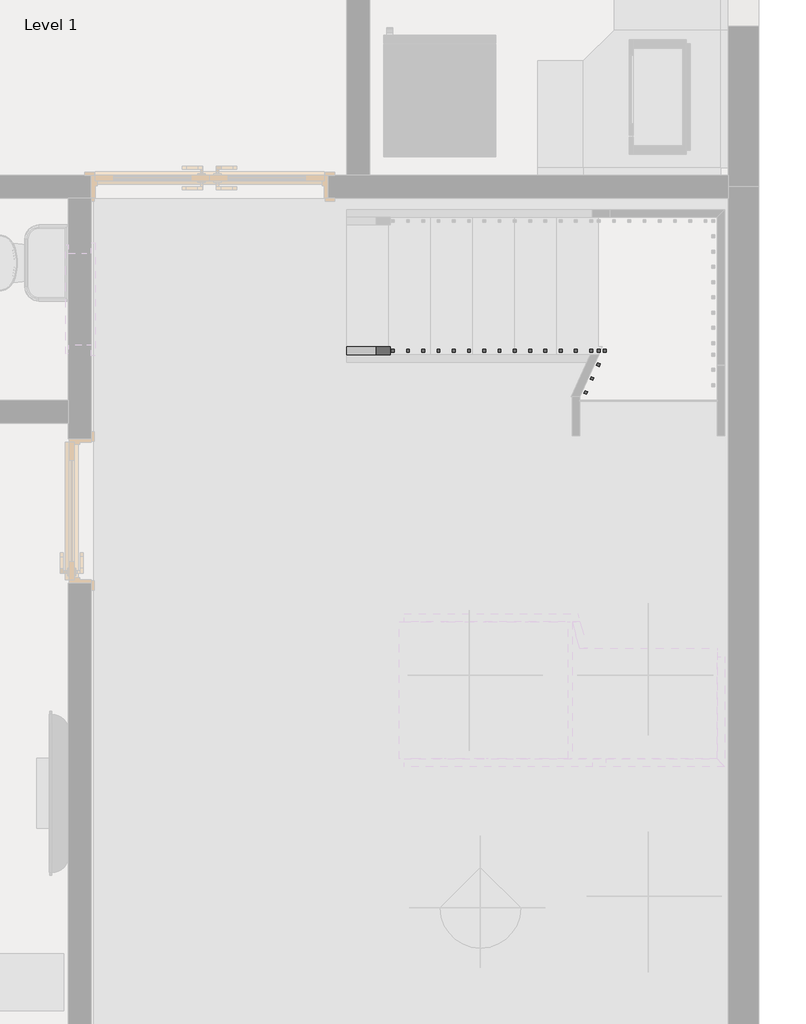
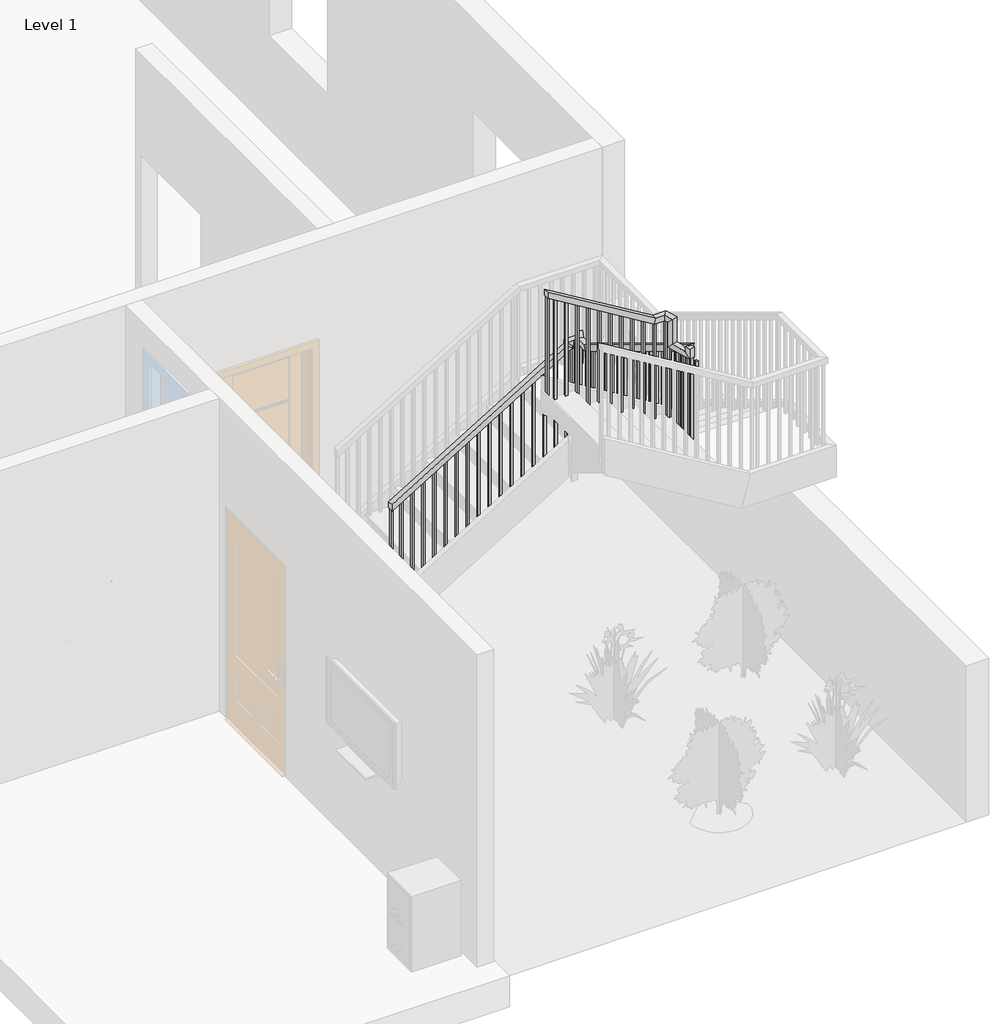
# One storey, part 2 of 4: 1 railing.
"""IFC4 building model written with IfcOpenShell, lengths in millimetres."""

from ifc_helpers import new_model, si_unit, frame, origin, place, context, project, spatial, polyline, outline, extrude, faceted_brep, element, save

model = new_model("IFC4")

# Units and contexts
model_context = context("Model", 3, world=origin())
ifc_project = project(units=[si_unit("LENGTHUNIT", "METRE", prefix="MILLI")], contexts=[model_context])

# Site, building, storey
site = spatial("IfcSite", under=ifc_project)
building = spatial("IfcBuilding", under=site)
storey = spatial("IfcBuildingStorey", under=building, Name="Level 1", Elevation=0.0)

# Railing
placement = place(None, origin())
element("IfcRailing", 1, ObjectType="Handrail - Rectangular", at=placement, inside=storey, context=model_context, shape_type="SolidModel", body=[
    faceted_brep([(-9231.9118598, 4390.9368529, 1083.7333333), (-9231.9118598, 4390.9368529, 1024.3318731), (-9231.9118598, 4340.1368529, 1024.3318731), (-9231.9118598, 4340.1368529, 1083.7333333), (-7617.6655536, 4390.9368529, 2062.064428), (-7566.8655536, 4390.9368529, 2033.4508465), (-7566.8655536, 4340.1368529, 2033.4508465), (-7617.6655536, 4340.1368529, 2062.064428), (-7617.6655536, 4390.9368529, 2099.7333333), (-7566.8655536, 4390.9368529, 2048.9333333), (-7566.8655536, 4340.1368529, 2048.9333333), (-7617.6655536, 4340.1368529, 2099.7333333), (-7476.6192475, 4390.9368529, 2099.7333333), (-7476.6192475, 4390.9368529, 2048.9333333), (-7555.5118598, 4340.1368529, 2048.9333333), (-7555.5118598, 4340.1368529, 2099.7333333), (-7534.9846242, 4262.533024, 2099.7333333), (-7534.9846242, 4262.533024, 2048.9333333), (-7581.2312413, 4283.5542135, 2048.9333333), (-7581.2312413, 4283.5542135, 2099.7333333), (-7591.9461721, 4137.2176186, 2099.7333333), (-7612.9673617, 4090.9710016, 2048.9333333), (-7659.2139787, 4111.9921912, 2048.9333333), (-7638.1927892, 4158.2388082, 2099.7333333), (-7591.9461721, 4137.2176186, 2333.9768931), (-7612.9673617, 4090.9710016, 2283.1768931), (-7659.2139787, 4111.9921912, 2283.1768931), (-7638.1927892, 4158.2388082, 2333.9768931), (-7631.7118598, 4049.7331058, 2333.9768931), (-7631.7118598, 4049.7331058, 2283.1768931), (-7682.5118598, 4060.7368529, 2283.1768931), (-7682.5118598, 4060.7368529, 2333.9768931), (-7631.7118598, 3953.6349793, 2333.9768931), (-7631.7118598, 3939.4425699, 2283.1768931), (-7682.5118598, 3939.4425699, 2283.1768931), (-7682.5118598, 3953.6349793, 2333.9768931), (-7631.7118598, 2279.1794573, 3348.7984216), (-7682.5118598, 2279.1794573, 3348.7984216), (-7682.5118598, 2329.9794573, 3258.6090825), (-7631.7118598, 2329.9794573, 3258.6090825)], [[[0, 1, 2, 3]], [[1, 0, 4, 5]], [[2, 1, 5, 6]], [[3, 2, 6, 7]], [[0, 3, 7, 4]], [[5, 4, 8, 9]], [[6, 5, 9, 10]], [[7, 6, 10, 11]], [[4, 7, 11, 8]], [[9, 8, 12, 13]], [[10, 9, 13, 14]], [[11, 10, 14, 15]], [[8, 11, 15, 12]], [[13, 12, 16, 17]], [[14, 13, 17, 18]], [[15, 14, 18, 19]], [[12, 15, 19, 16]], [[17, 16, 20, 21]], [[18, 17, 21, 22]], [[19, 18, 22, 23]], [[16, 19, 23, 20]], [[21, 20, 24, 25]], [[22, 21, 25, 26]], [[23, 22, 26, 27]], [[20, 23, 27, 24]], [[25, 24, 28, 29]], [[26, 25, 29, 30]], [[27, 26, 30, 31]], [[24, 27, 31, 28]], [[29, 28, 32, 33]], [[30, 29, 33, 34]], [[31, 30, 34, 35]], [[28, 31, 35, 32]], [[36, 37, 38, 39]], [[33, 32, 36, 39]], [[34, 33, 39, 38]], [[35, 34, 38, 37]], [[32, 35, 37, 36]]]),
    faceted_brep([(-7709.4462346, 2293.6923737, 3333.4044822), (-7695.4904013, 2244.8469572, 3333.4044822), (-7646.6449848, 2258.8027905, 3333.4044822), (-7660.6008181, 2307.648207, 3333.4044822), (-7709.4462346, 2293.6923737, 3285.0666667), (-7695.4904013, 2244.8469572, 3234.2666667), (-7646.6449848, 2258.8027905, 3234.2666667), (-7660.6008181, 2307.648207, 3285.0666667), (-7748.9821573, 2432.0681031, 3285.0666667), (-7762.9379906, 2480.9135197, 3234.2666667), (-7714.0925741, 2494.869353, 3234.2666667), (-7700.1367408, 2446.0239364, 3285.0666667), (-7748.9821573, 2432.0681031, 3527.5874278), (-7762.9379906, 2480.9135197, 3476.7874278), (-7714.0925741, 2494.869353, 3476.7874278), (-7700.1367408, 2446.0239364, 3527.5874278), (-7771.6303715, 2511.3368529, 3527.5874278), (-7771.6303715, 2511.3368529, 3476.7874278), (-7733.3118598, 2562.1368529, 3476.7874278), (-7733.3118598, 2562.1368529, 3527.5874278), (-7854.0711157, 2511.3368529, 3527.5874278), (-7868.2635251, 2511.3368529, 3476.7874278), (-7868.2635251, 2562.1368529, 3476.7874278), (-7854.0711157, 2562.1368529, 3527.5874278), (-8850.9118598, 2511.3368529, 4131.7333333), (-8850.9118598, 2562.1368529, 4131.7333333), (-8850.9118598, 2562.1368529, 4072.3318731), (-8850.9118598, 2511.3368529, 4072.3318731)], [[[0, 1, 2, 3]], [[1, 0, 4, 5]], [[2, 1, 5, 6]], [[3, 2, 6, 7]], [[0, 3, 7, 4]], [[5, 4, 8, 9]], [[6, 5, 9, 10]], [[7, 6, 10, 11]], [[4, 7, 11, 8]], [[9, 8, 12, 13]], [[10, 9, 13, 14]], [[11, 10, 14, 15]], [[8, 11, 15, 12]], [[13, 12, 16, 17]], [[14, 13, 17, 18]], [[15, 14, 18, 19]], [[12, 15, 19, 16]], [[17, 16, 20, 21]], [[18, 17, 21, 22]], [[19, 18, 22, 23]], [[16, 19, 23, 20]], [[24, 25, 26, 27]], [[21, 20, 24, 27]], [[22, 21, 27, 26]], [[23, 22, 26, 25]], [[20, 23, 25, 24]]]),
    extrude(outline(polyline([(4016.5950585, -8758.9461157), (4028.140513, -8777.9961157), (3048.0, -8777.9961157), (3048.0, -8758.9461157), (4016.5950585, -8758.9461157)])), frame((0.0, 2527.2118529, 0.0), z_axis=(0.0, 1.0, 0.0), x_axis=(0.0, 0.0, 1.0)), (0.0, 0.0, 1.0), 19.05),
    extrude(outline(polyline([(3955.0193009, -8657.3461157), (3966.5647554, -8676.3961157), (3048.0, -8676.3961157), (3048.0, -8657.3461157), (3955.0193009, -8657.3461157)])), frame((0.0, 2527.2118529, 0.0), z_axis=(0.0, 1.0, 0.0), x_axis=(0.0, 0.0, 1.0)), (0.0, 0.0, 1.0), 19.05),
    extrude(outline(polyline([(3893.4435433, -8555.7461157), (3904.9889979, -8574.7961157), (2878.6666667, -8574.7961157), (2878.6666667, -8555.7461157), (3893.4435433, -8555.7461157)])), frame((0.0, 2527.2118529, 0.0), z_axis=(0.0, 1.0, 0.0), x_axis=(0.0, 0.0, 1.0)), (0.0, 0.0, 1.0), 19.05),
    extrude(outline(polyline([(3831.8677857, -8454.1461157), (3843.4132403, -8473.1961157), (2878.6666667, -8473.1961157), (2878.6666667, -8454.1461157), (3831.8677857, -8454.1461157)])), frame((0.0, 2527.2118529, 0.0), z_axis=(0.0, 1.0, 0.0), x_axis=(0.0, 0.0, 1.0)), (0.0, 0.0, 1.0), 19.05),
    extrude(outline(polyline([(3770.2920282, -8352.5461157), (3781.8374827, -8371.5961157), (2878.6666667, -8371.5961157), (2878.6666667, -8352.5461157), (3770.2920282, -8352.5461157)])), frame((0.0, 2527.2118529, 0.0), z_axis=(0.0, 1.0, 0.0), x_axis=(0.0, 0.0, 1.0)), (0.0, 0.0, 1.0), 19.05),
    extrude(outline(polyline([(3708.7162706, -8250.9461157), (3720.2617251, -8269.9961157), (2709.3333333, -8269.9961157), (2709.3333333, -8250.9461157), (3708.7162706, -8250.9461157)])), frame((0.0, 2527.2118529, 0.0), z_axis=(0.0, 1.0, 0.0), x_axis=(0.0, 0.0, 1.0)), (0.0, 0.0, 1.0), 19.05),
    extrude(outline(polyline([(3647.140513, -8149.3461157), (3658.6859676, -8168.3961157), (2709.3333333, -8168.3961157), (2709.3333333, -8149.3461157), (3647.140513, -8149.3461157)])), frame((0.0, 2527.2118529, 0.0), z_axis=(0.0, 1.0, 0.0), x_axis=(0.0, 0.0, 1.0)), (0.0, 0.0, 1.0), 19.05),
    extrude(outline(polyline([(3585.5647554, -8047.7461157), (3597.11021, -8066.7961157), (2709.3333333, -8066.7961157), (2709.3333333, -8047.7461157), (3585.5647554, -8047.7461157)])), frame((0.0, 2527.2118529, 0.0), z_axis=(0.0, 1.0, 0.0), x_axis=(0.0, 0.0, 1.0)), (0.0, 0.0, 1.0), 19.05),
    extrude(outline(polyline([(3523.9889979, -7946.1461157), (3535.5344524, -7965.1961157), (2540.0, -7965.1961157), (2540.0, -7946.1461157), (3523.9889979, -7946.1461157)])), frame((0.0, 2527.2118529, 0.0), z_axis=(0.0, 1.0, 0.0), x_axis=(0.0, 0.0, 1.0)), (0.0, 0.0, 1.0), 19.05),
    extrude(outline(polyline([(-7844.5461157, 2546.2618529), (-7844.5461157, 2527.2118529), (-7863.5961157, 2527.2118529), (-7863.5961157, 2546.2618529), (-7844.5461157, 2546.2618529)])), frame((0.0, 0.0, 2540.0), z_axis=(0.0, 0.0, 1.0), x_axis=(1.0, 0.0, 0.0)), (0.0, 0.0, 1.0), 936.7874278),
    extrude(outline(polyline([(-7729.0716252, 2489.5101597), (-7747.3886564, 2484.2767222), (-7752.6220939, 2502.5937534), (-7734.3050627, 2507.8271909), (-7729.0716252, 2489.5101597)])), frame((0.0, 0.0, 2540.0), z_axis=(0.0, 0.0, 1.0), x_axis=(1.0, 0.0, 0.0)), (0.0, 0.0, 1.0), 694.2666667),
    extrude(outline(polyline([(-7701.1599586, 2391.8193266), (-7719.4769898, 2386.5858891), (-7724.7104273, 2404.9029203), (-7706.3933961, 2410.1363578), (-7701.1599586, 2391.8193266)])), frame((0.0, 0.0, 2370.6666667), z_axis=(0.0, 0.0, 1.0), x_axis=(1.0, 0.0, 0.0)), (0.0, 0.0, 1.0), 863.6),
    extrude(outline(polyline([(-7673.248292, 2294.1284935), (-7691.5653232, 2288.895056), (-7696.7987607, 2307.2120872), (-7678.4817295, 2312.4455247), (-7673.248292, 2294.1284935)])), frame((0.0, 0.0, 2370.6666667), z_axis=(0.0, 0.0, 1.0), x_axis=(1.0, 0.0, 0.0)), (0.0, 0.0, 1.0), 863.6),
    extrude(outline(polyline([(-7666.6368598, 2292.2618529), (-7647.5868598, 2292.2618529), (-7647.5868598, 2273.2118529), (-7666.6368598, 2273.2118529), (-7666.6368598, 2292.2618529)])), frame((0.0, 0.0, 2370.6666667), z_axis=(0.0, 0.0, 1.0), x_axis=(1.0, 0.0, 0.0)), (0.0, 0.0, 1.0), 863.6),
    extrude(outline(polyline([(2420.1099793, 3203.9845237), (2439.1599793, 3192.4390692), (2439.1599793, 2201.3333333), (2420.1099793, 2201.3333333), (2420.1099793, 3203.9845237)])), frame((-7666.6368598, 0.0, 0.0), z_axis=(1.0, 0.0, 0.0), x_axis=(0.0, 1.0, 0.0)), (0.0, 0.0, 1.0), 19.05),
    extrude(outline(polyline([(2521.7099793, 3142.4087661), (2540.7599793, 3130.8633116), (2540.7599793, 2201.3333333), (2521.7099793, 2201.3333333), (2521.7099793, 3142.4087661)])), frame((-7666.6368598, 0.0, 0.0), z_axis=(1.0, 0.0, 0.0), x_axis=(0.0, 1.0, 0.0)), (0.0, 0.0, 1.0), 19.05),
    extrude(outline(polyline([(2623.3099793, 3080.8330086), (2642.3599793, 3069.287554), (2642.3599793, 2201.3333333), (2623.3099793, 2201.3333333), (2623.3099793, 3080.8330086)])), frame((-7666.6368598, 0.0, 0.0), z_axis=(1.0, 0.0, 0.0), x_axis=(0.0, 1.0, 0.0)), (0.0, 0.0, 1.0), 19.05),
    extrude(outline(polyline([(2724.9099793, 3019.257251), (2743.9599793, 3007.7117964), (2743.9599793, 2032.0), (2724.9099793, 2032.0), (2724.9099793, 3019.257251)])), frame((-7666.6368598, 0.0, 0.0), z_axis=(1.0, 0.0, 0.0), x_axis=(0.0, 1.0, 0.0)), (0.0, 0.0, 1.0), 19.05),
    extrude(outline(polyline([(2826.5099793, 2957.6814934), (2845.5599793, 2946.1360389), (2845.5599793, 2032.0), (2826.5099793, 2032.0), (2826.5099793, 2957.6814934)])), frame((-7666.6368598, 0.0, 0.0), z_axis=(1.0, 0.0, 0.0), x_axis=(0.0, 1.0, 0.0)), (0.0, 0.0, 1.0), 19.05),
    extrude(outline(polyline([(2928.1099793, 2896.1057358), (2947.1599793, 2884.5602813), (2947.1599793, 2032.0), (2928.1099793, 2032.0), (2928.1099793, 2896.1057358)])), frame((-7666.6368598, 0.0, 0.0), z_axis=(1.0, 0.0, 0.0), x_axis=(0.0, 1.0, 0.0)), (0.0, 0.0, 1.0), 19.05),
    extrude(outline(polyline([(3029.7099793, 2834.5299783), (3048.7599793, 2822.9845237), (3048.7599793, 1862.6666667), (3029.7099793, 1862.6666667), (3029.7099793, 2834.5299783)])), frame((-7666.6368598, 0.0, 0.0), z_axis=(1.0, 0.0, 0.0), x_axis=(0.0, 1.0, 0.0)), (0.0, 0.0, 1.0), 19.05),
    extrude(outline(polyline([(3131.3099793, 2772.9542207), (3150.3599793, 2761.4087661), (3150.3599793, 1862.6666667), (3131.3099793, 1862.6666667), (3131.3099793, 2772.9542207)])), frame((-7666.6368598, 0.0, 0.0), z_axis=(1.0, 0.0, 0.0), x_axis=(0.0, 1.0, 0.0)), (0.0, 0.0, 1.0), 19.05),
    extrude(outline(polyline([(3232.9099793, 2711.3784631), (3251.9599793, 2699.8330086), (3251.9599793, 1693.3333333), (3232.9099793, 1693.3333333), (3232.9099793, 2711.3784631)])), frame((-7666.6368598, 0.0, 0.0), z_axis=(1.0, 0.0, 0.0), x_axis=(0.0, 1.0, 0.0)), (0.0, 0.0, 1.0), 19.05),
    extrude(outline(polyline([(3334.5099793, 2649.8027055), (3353.5599793, 2638.257251), (3353.5599793, 1693.3333333), (3334.5099793, 1693.3333333), (3334.5099793, 2649.8027055)])), frame((-7666.6368598, 0.0, 0.0), z_axis=(1.0, 0.0, 0.0), x_axis=(0.0, 1.0, 0.0)), (0.0, 0.0, 1.0), 19.05),
    extrude(outline(polyline([(3436.1099793, 2588.226948), (3455.1599793, 2576.6814934), (3455.1599793, 1693.3333333), (3436.1099793, 1693.3333333), (3436.1099793, 2588.226948)])), frame((-7666.6368598, 0.0, 0.0), z_axis=(1.0, 0.0, 0.0), x_axis=(0.0, 1.0, 0.0)), (0.0, 0.0, 1.0), 19.05),
    extrude(outline(polyline([(3537.7099793, 2526.6511904), (3556.7599793, 2515.1057358), (3556.7599793, 1524.0), (3537.7099793, 1524.0), (3537.7099793, 2526.6511904)])), frame((-7666.6368598, 0.0, 0.0), z_axis=(1.0, 0.0, 0.0), x_axis=(0.0, 1.0, 0.0)), (0.0, 0.0, 1.0), 19.05),
    extrude(outline(polyline([(3639.3099793, 2465.0754328), (3658.3599793, 2453.5299783), (3658.3599793, 1524.0), (3639.3099793, 1524.0), (3639.3099793, 2465.0754328)])), frame((-7666.6368598, 0.0, 0.0), z_axis=(1.0, 0.0, 0.0), x_axis=(0.0, 1.0, 0.0)), (0.0, 0.0, 1.0), 19.05),
    extrude(outline(polyline([(3740.9099793, 2403.4996752), (3759.9599793, 2391.9542207), (3759.9599793, 1524.0), (3740.9099793, 1524.0), (3740.9099793, 2403.4996752)])), frame((-7666.6368598, 0.0, 0.0), z_axis=(1.0, 0.0, 0.0), x_axis=(0.0, 1.0, 0.0)), (0.0, 0.0, 1.0), 19.05),
    extrude(outline(polyline([(3842.5099793, 2341.9239177), (3861.5599793, 2330.3784631), (3861.5599793, 1354.6666667), (3842.5099793, 1354.6666667), (3842.5099793, 2341.9239177)])), frame((-7666.6368598, 0.0, 0.0), z_axis=(1.0, 0.0, 0.0), x_axis=(0.0, 1.0, 0.0)), (0.0, 0.0, 1.0), 19.05),
    extrude(outline(polyline([(-7666.6368598, 3963.1599793), (-7647.5868598, 3963.1599793), (-7647.5868598, 3944.1099793), (-7666.6368598, 3944.1099793), (-7666.6368598, 3963.1599793)])), frame((0.0, 0.0, 1354.6666667), z_axis=(0.0, 0.0, 1.0), x_axis=(1.0, 0.0, 0.0)), (0.0, 0.0, 1.0), 928.5102264),
    extrude(outline(polyline([(-7646.9224587, 4100.6698643), (-7629.5799773, 4092.7869182), (-7637.4629234, 4075.4444368), (-7654.8054048, 4083.3273829), (-7646.9224587, 4100.6698643)])), frame((0.0, 0.0, 1185.3333333), z_axis=(0.0, 0.0, 1.0), x_axis=(1.0, 0.0, 0.0)), (0.0, 0.0, 1.0), 1097.8435597),
    extrude(outline(polyline([(-7604.8800796, 4193.1630984), (-7587.5375982, 4185.2801523), (-7595.4205443, 4167.9376709), (-7612.7630256, 4175.820617), (-7604.8800796, 4193.1630984)])), frame((0.0, 0.0, 1185.3333333), z_axis=(0.0, 0.0, 1.0), x_axis=(1.0, 0.0, 0.0)), (0.0, 0.0, 1.0), 863.6),
    extrude(outline(polyline([(-7562.8377004, 4285.6563325), (-7545.495219, 4277.7733864), (-7553.3781651, 4260.430905), (-7570.7206465, 4268.3138511), (-7562.8377004, 4285.6563325)])), frame((0.0, 0.0, 1185.3333333), z_axis=(0.0, 0.0, 1.0), x_axis=(1.0, 0.0, 0.0)), (0.0, 0.0, 1.0), 863.6),
    extrude(outline(polyline([(2015.3167216, -7596.7868598), (2003.771267, -7615.8368598), (1016.0, -7615.8368598), (1016.0, -7596.7868598), (2015.3167216, -7596.7868598)])), frame((0.0, 4356.0118529, 0.0), z_axis=(0.0, 1.0, 0.0), x_axis=(0.0, 0.0, 1.0)), (0.0, 0.0, 1.0), 19.05),
    extrude(outline(polyline([(1953.740964, -7698.3868598), (1942.1955094, -7717.4368598), (1016.0, -7717.4368598), (1016.0, -7698.3868598), (1953.740964, -7698.3868598)])), frame((0.0, 4356.0118529, 0.0), z_axis=(0.0, 1.0, 0.0), x_axis=(0.0, 0.0, 1.0)), (0.0, 0.0, 1.0), 19.05),
    extrude(outline(polyline([(1892.1652064, -7799.9868598), (1880.6197519, -7819.0368598), (1016.0, -7819.0368598), (1016.0, -7799.9868598), (1892.1652064, -7799.9868598)])), frame((0.0, 4356.0118529, 0.0), z_axis=(0.0, 1.0, 0.0), x_axis=(0.0, 0.0, 1.0)), (0.0, 0.0, 1.0), 19.05),
    extrude(outline(polyline([(1830.5894488, -7901.5868598), (1819.0439943, -7920.6368598), (846.6666667, -7920.6368598), (846.6666667, -7901.5868598), (1830.5894488, -7901.5868598)])), frame((0.0, 4356.0118529, 0.0), z_axis=(0.0, 1.0, 0.0), x_axis=(0.0, 0.0, 1.0)), (0.0, 0.0, 1.0), 19.05),
    extrude(outline(polyline([(1769.0136913, -8003.1868598), (1757.4682367, -8022.2368598), (846.6666667, -8022.2368598), (846.6666667, -8003.1868598), (1769.0136913, -8003.1868598)])), frame((0.0, 4356.0118529, 0.0), z_axis=(0.0, 1.0, 0.0), x_axis=(0.0, 0.0, 1.0)), (0.0, 0.0, 1.0), 19.05),
    extrude(outline(polyline([(1707.4379337, -8104.7868598), (1695.8924791, -8123.8368598), (846.6666667, -8123.8368598), (846.6666667, -8104.7868598), (1707.4379337, -8104.7868598)])), frame((0.0, 4356.0118529, 0.0), z_axis=(0.0, 1.0, 0.0), x_axis=(0.0, 0.0, 1.0)), (0.0, 0.0, 1.0), 19.05),
    extrude(outline(polyline([(1645.8621761, -8206.3868598), (1634.3167216, -8225.4368598), (677.3333333, -8225.4368598), (677.3333333, -8206.3868598), (1645.8621761, -8206.3868598)])), frame((0.0, 4356.0118529, 0.0), z_axis=(0.0, 1.0, 0.0), x_axis=(0.0, 0.0, 1.0)), (0.0, 0.0, 1.0), 19.05),
    extrude(outline(polyline([(1584.2864185, -8307.9868598), (1572.740964, -8327.0368598), (677.3333333, -8327.0368598), (677.3333333, -8307.9868598), (1584.2864185, -8307.9868598)])), frame((0.0, 4356.0118529, 0.0), z_axis=(0.0, 1.0, 0.0), x_axis=(0.0, 0.0, 1.0)), (0.0, 0.0, 1.0), 19.05),
    extrude(outline(polyline([(1522.710661, -8409.5868598), (1511.1652064, -8428.6368598), (508.0, -8428.6368598), (508.0, -8409.5868598), (1522.710661, -8409.5868598)])), frame((0.0, 4356.0118529, 0.0), z_axis=(0.0, 1.0, 0.0), x_axis=(0.0, 0.0, 1.0)), (0.0, 0.0, 1.0), 19.05),
    extrude(outline(polyline([(1461.1349034, -8511.1868598), (1449.5894488, -8530.2368598), (508.0, -8530.2368598), (508.0, -8511.1868598), (1461.1349034, -8511.1868598)])), frame((0.0, 4356.0118529, 0.0), z_axis=(0.0, 1.0, 0.0), x_axis=(0.0, 0.0, 1.0)), (0.0, 0.0, 1.0), 19.05),
    extrude(outline(polyline([(1399.5591458, -8612.7868598), (1388.0136913, -8631.8368598), (508.0, -8631.8368598), (508.0, -8612.7868598), (1399.5591458, -8612.7868598)])), frame((0.0, 4356.0118529, 0.0), z_axis=(0.0, 1.0, 0.0), x_axis=(0.0, 0.0, 1.0)), (0.0, 0.0, 1.0), 19.05),
    extrude(outline(polyline([(1337.9833882, -8714.3868598), (1326.4379337, -8733.4368598), (338.6666667, -8733.4368598), (338.6666667, -8714.3868598), (1337.9833882, -8714.3868598)])), frame((0.0, 4356.0118529, 0.0), z_axis=(0.0, 1.0, 0.0), x_axis=(0.0, 0.0, 1.0)), (0.0, 0.0, 1.0), 19.05),
    extrude(outline(polyline([(1276.4076307, -8815.9868598), (1264.8621761, -8835.0368598), (338.6666667, -8835.0368598), (338.6666667, -8815.9868598), (1276.4076307, -8815.9868598)])), frame((0.0, 4356.0118529, 0.0), z_axis=(0.0, 1.0, 0.0), x_axis=(0.0, 0.0, 1.0)), (0.0, 0.0, 1.0), 19.05),
    extrude(outline(polyline([(1214.8318731, -8917.5868598), (1203.2864185, -8936.6368598), (338.6666667, -8936.6368598), (338.6666667, -8917.5868598), (1214.8318731, -8917.5868598)])), frame((0.0, 4356.0118529, 0.0), z_axis=(0.0, 1.0, 0.0), x_axis=(0.0, 0.0, 1.0)), (0.0, 0.0, 1.0), 19.05),
    extrude(outline(polyline([(1153.2561155, -9019.1868598), (1141.710661, -9038.2368598), (169.3333333, -9038.2368598), (169.3333333, -9019.1868598), (1153.2561155, -9019.1868598)])), frame((0.0, 4356.0118529, 0.0), z_axis=(0.0, 1.0, 0.0), x_axis=(0.0, 0.0, 1.0)), (0.0, 0.0, 1.0), 19.05),
    extrude(outline(polyline([(1091.6803579, -9120.7868598), (1080.1349034, -9139.8368598), (169.3333333, -9139.8368598), (169.3333333, -9120.7868598), (1091.6803579, -9120.7868598)])), frame((0.0, 4356.0118529, 0.0), z_axis=(0.0, 1.0, 0.0), x_axis=(0.0, 0.0, 1.0)), (0.0, 0.0, 1.0), 19.05),
    extrude(outline(polyline([(-7742.9461157, 2546.2618529), (-7742.9461157, 2527.2118529), (-7761.9961157, 2527.2118529), (-7761.9961157, 2546.2618529), (-7742.9461157, 2546.2618529)])), frame((0.0, 0.0, 2540.0), z_axis=(0.0, 0.0, 1.0), x_axis=(1.0, 0.0, 0.0)), (0.0, 0.0, 1.0), 936.7874278),
    extrude(outline(polyline([(-7666.6368598, 2212.5044573), (-7647.5868598, 2212.5044573), (-7647.5868598, 2193.4544573), (-7666.6368598, 2193.4544573), (-7666.6368598, 2212.5044573)])), frame((0.0, 0.0, 2370.6666667), z_axis=(0.0, 0.0, 1.0), x_axis=(1.0, 0.0, 0.0)), (0.0, 0.0, 1.0), 863.6),
    extrude(outline(polyline([(2374.8118529, 3231.4379337), (2393.8618529, 3219.8924791), (2393.8618529, 2370.6666667), (2374.8118529, 2370.6666667), (2374.8118529, 3231.4379337)])), frame((-7666.6368598, 0.0, 0.0), z_axis=(1.0, 0.0, 0.0), x_axis=(0.0, 1.0, 0.0)), (0.0, 0.0, 1.0), 19.05),
    extrude(outline(polyline([(-7666.6368598, 4064.7599793), (-7647.5868598, 4064.7599793), (-7647.5868598, 4045.7099793), (-7666.6368598, 4045.7099793), (-7666.6368598, 4064.7599793)])), frame((0.0, 0.0, 1354.6666667), z_axis=(0.0, 0.0, 1.0), x_axis=(1.0, 0.0, 0.0)), (0.0, 0.0, 1.0), 928.5102264),
    extrude(outline(polyline([(-7525.5905536, 4356.0118529), (-7525.5905536, 4375.0618529), (-7506.5405536, 4375.0618529), (-7506.5405536, 4356.0118529), (-7525.5905536, 4356.0118529)])), frame((0.0, 0.0, 1185.3333333), z_axis=(0.0, 0.0, 1.0), x_axis=(1.0, 0.0, 0.0)), (0.0, 0.0, 1.0), 863.6),
    extrude(outline(polyline([(-7565.0368598, 4356.0118529), (-7565.0368598, 4375.0618529), (-7545.9868598, 4375.0618529), (-7545.9868598, 4356.0118529), (-7565.0368598, 4356.0118529)])), frame((0.0, 0.0, 1185.3333333), z_axis=(0.0, 0.0, 1.0), x_axis=(1.0, 0.0, 0.0)), (0.0, 0.0, 1.0), 825.9310946),
    extrude(outline(polyline([(4060.7864185, -8831.8618598), (4072.3318731, -8850.9118598), (3048.0, -8850.9118598), (3048.0, -8831.8618598), (4060.7864185, -8831.8618598)])), frame((0.0, 2527.2118529, 0.0), z_axis=(0.0, 1.0, 0.0), x_axis=(0.0, 0.0, 1.0)), (0.0, 0.0, 1.0), 19.05),
    extrude(outline(polyline([(1035.8773276, -9212.8618598), (1024.3318731, -9231.9118598), (169.3333333, -9231.9118598), (169.3333333, -9212.8618598), (1035.8773276, -9212.8618598)])), frame((0.0, 4356.0118529, 0.0), z_axis=(0.0, 1.0, 0.0), x_axis=(0.0, 0.0, 1.0)), (0.0, 0.0, 1.0), 19.05),
])

save(model, "model.ifc")

# Revit data of these elements
# Type "Handrail - Rectangular"
#   Assembly Code = "C2010400"
#   built-in parameter 1008612 = 0.0416667 (stored number, unit not read)
#   built-in parameter 1008611 = 0.0416667 (stored number, unit not read)
#   built-in parameter 1008609 = 0.333333 (stored number, unit not read)
#   built-in parameter 1008604 = 0.166667 (stored number, unit not read)
#   built-in parameter 1008603 = 0.166667 (stored number, unit not read)
#   Railing Height = 3' - 0"
#   built-in parameter 1008630 = 2
#   built-in parameter 1008610 = 2
#   built-in parameter 1008618 = Baluster - Square : 3/4"
# Element 1 (IfcRailing, "Handrail - Rectangular")
#   Phase Created = New Construction
